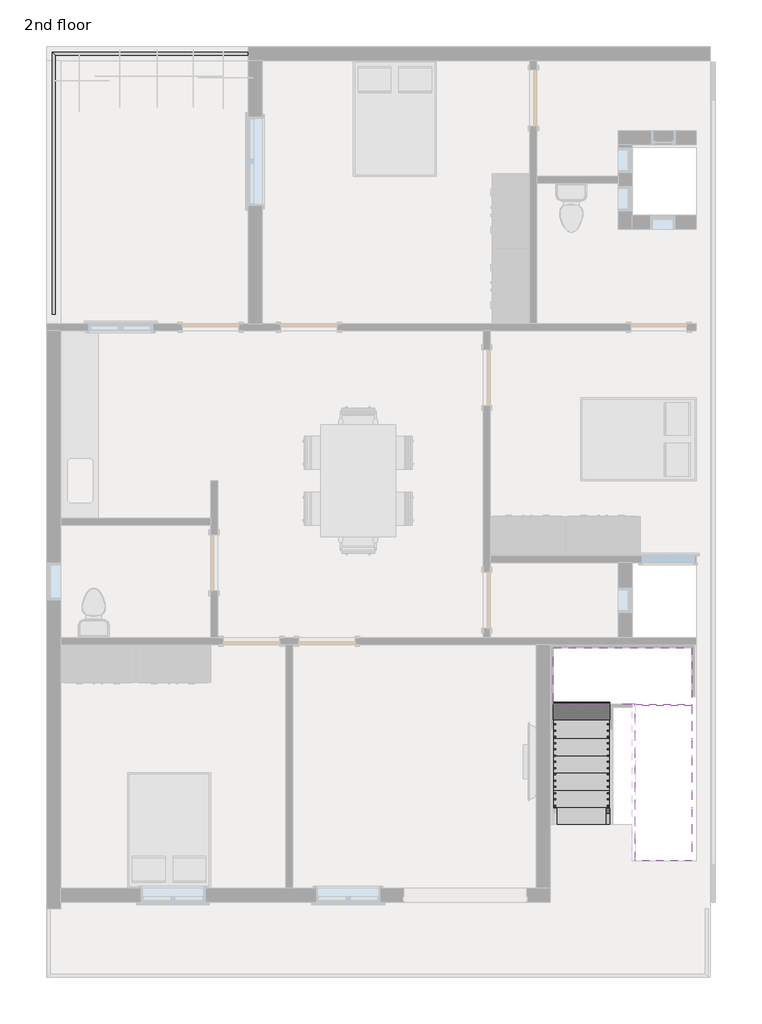
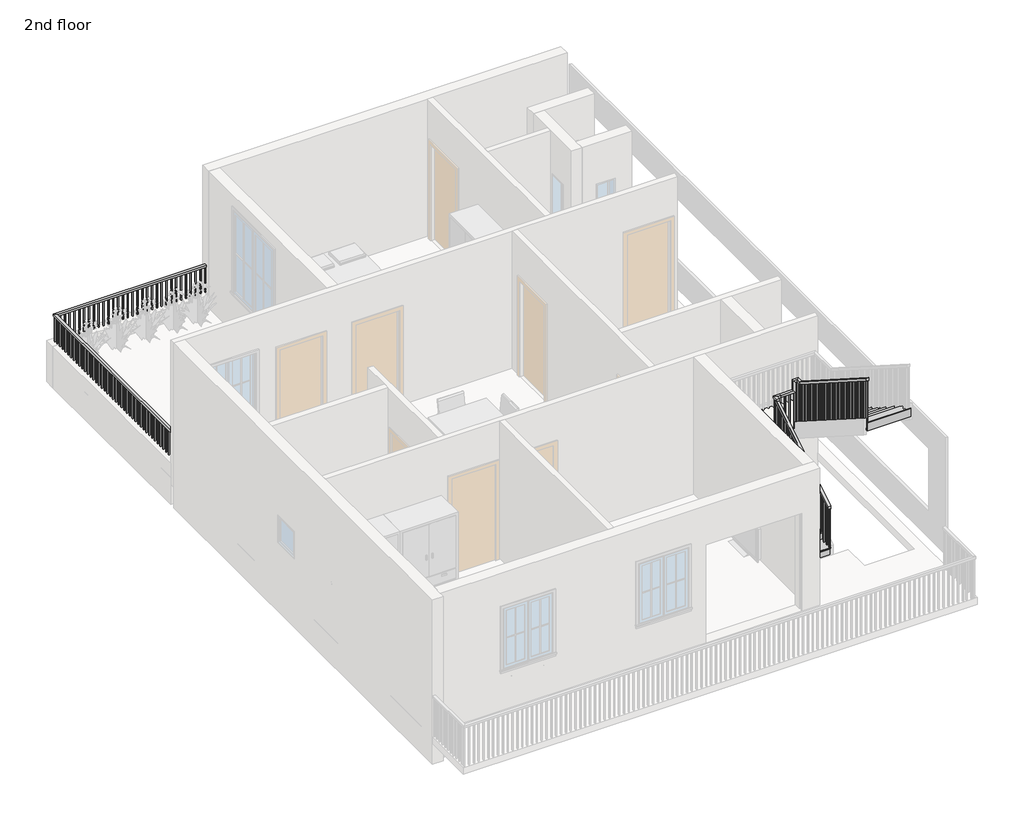
# One storey, part 3 of 5: 2 railings, 2 stair flights, 1 slab.
"""IFC4 building model written with IfcOpenShell, lengths in millimetres."""

from ifc_helpers import new_model, si_unit, frame, origin, place, context, project, spatial, polyline, outline, extrude, faceted_brep, transform, mapped, element, save
from components import non_monolithic_landing_99b9b51a, stair_flight_e21d000d, stair_flight_364c9dde

model = new_model("IFC4")

# Units and contexts
model_context = context("Model", 3, world=origin())
ifc_project = project(units=[si_unit("LENGTHUNIT", "METRE", prefix="MILLI")], contexts=[model_context])

# Site, building, storey
site = spatial("IfcSite", under=ifc_project)
building = spatial("IfcBuilding", under=site)
storey = spatial("IfcBuildingStorey", under=building, Name="2nd floor", Elevation=7010.4)

# Railings
placement = place(None, origin())
element("IfcRailing", 1, ObjectType="Handrail - Rectangular", at=placement, inside=storey, context=model_context, shape_type="SolidModel", body=[
    faceted_brep([(995.5501403, 157.6257925, 8102.6), (995.5501403, 157.6257925, 8042.386276), (1046.3501403, 157.6257925, 8042.386276), (1046.3501403, 157.6257925, 8102.6), (995.5501403, 2037.2257925, 9298.7090909), (995.5501403, 2088.0257925, 9270.8226396), (1046.3501403, 2088.0257925, 9270.8226396), (1046.3501403, 2037.2257925, 9298.7090909), (995.5501403, 2037.2257925, 9347.2), (995.5501403, 2088.0257925, 9296.4), (1046.3501403, 2088.0257925, 9296.4), (1046.3501403, 2037.2257925, 9347.2), (995.5501403, 2164.2257925, 9347.2), (995.5501403, 2164.2257925, 9296.4), (1046.3501403, 2113.4257925, 9296.4), (1046.3501403, 2113.4257925, 9347.2), (1122.5501403, 2164.2257925, 9347.2), (1122.5501403, 2164.2257925, 9296.4), (1122.5501403, 2113.4257925, 9296.4), (1122.5501403, 2113.4257925, 9347.2), (1389.2501403, 2164.2257925, 9347.2), (1440.0501403, 2164.2257925, 9296.4), (1440.0501403, 2113.4257925, 9296.4), (1389.2501403, 2113.4257925, 9347.2), (1389.2501403, 2164.2257925, 9573.4909091), (1440.0501403, 2164.2257925, 9522.6909091), (1440.0501403, 2113.4257925, 9522.6909091), (1389.2501403, 2113.4257925, 9573.4909091), (1516.2501403, 2164.2257925, 9573.4909091), (1516.2501403, 2164.2257925, 9522.6909091), (1465.4501403, 2113.4257925, 9522.6909091), (1465.4501403, 2113.4257925, 9573.4909091), (1516.2501403, 2037.2257925, 9573.4909091), (1516.2501403, 2022.4327976, 9522.6909091), (1465.4501403, 2022.4327976, 9522.6909091), (1465.4501403, 2037.2257925, 9573.4909091), (1516.2501403, -401.1742075, 11125.2), (1465.4501403, -401.1742075, 11125.2), (1465.4501403, -401.1742075, 11064.986276), (1516.2501403, -401.1742075, 11064.986276)], [[[0, 1, 2, 3]], [[1, 0, 4, 5]], [[2, 1, 5, 6]], [[3, 2, 6, 7]], [[0, 3, 7, 4]], [[5, 4, 8, 9]], [[6, 5, 9, 10]], [[7, 6, 10, 11]], [[4, 7, 11, 8]], [[9, 8, 12, 13]], [[10, 9, 13, 14]], [[11, 10, 14, 15]], [[8, 11, 15, 12]], [[13, 12, 16, 17]], [[14, 13, 17, 18]], [[15, 14, 18, 19]], [[12, 15, 19, 16]], [[17, 16, 20, 21]], [[18, 17, 21, 22]], [[19, 18, 22, 23]], [[16, 19, 23, 20]], [[21, 20, 24, 25]], [[22, 21, 25, 26]], [[23, 22, 26, 27]], [[20, 23, 27, 24]], [[25, 24, 28, 29]], [[26, 25, 29, 30]], [[27, 26, 30, 31]], [[24, 27, 31, 28]], [[29, 28, 32, 33]], [[30, 29, 33, 34]], [[31, 30, 34, 35]], [[28, 31, 35, 32]], [[36, 37, 38, 39]], [[33, 32, 36, 39]], [[34, 33, 39, 38]], [[35, 34, 38, 37]], [[32, 35, 37, 36]]]),
    extrude(outline(polyline([(-309.0992075, 11006.3930941), (-290.0492075, 10994.2703669), (-290.0492075, 10033.0), (-309.0992075, 10033.0), (-309.0992075, 11006.3930941)])), frame((1481.3251403, 0.0, 0.0), z_axis=(1.0, 0.0, 0.0), x_axis=(0.0, 1.0, 0.0)), (0.0, 0.0, 1.0), 19.05),
    extrude(outline(polyline([(-207.4992075, 10941.7385487), (-188.4492075, 10929.6158214), (-188.4492075, 10033.0), (-207.4992075, 10033.0), (-207.4992075, 10941.7385487)])), frame((1481.3251403, 0.0, 0.0), z_axis=(1.0, 0.0, 0.0), x_axis=(0.0, 1.0, 0.0)), (0.0, 0.0, 1.0), 19.05),
    extrude(outline(polyline([(-105.8992075, 10877.0840032), (-86.8492075, 10864.961276), (-86.8492075, 9855.2), (-105.8992075, 9855.2), (-105.8992075, 10877.0840032)])), frame((1481.3251403, 0.0, 0.0), z_axis=(1.0, 0.0, 0.0), x_axis=(0.0, 1.0, 0.0)), (0.0, 0.0, 1.0), 19.05),
    extrude(outline(polyline([(-4.2992075, 10812.4294578), (14.7507925, 10800.3067305), (14.7507925, 9855.2), (-4.2992075, 9855.2), (-4.2992075, 10812.4294578)])), frame((1481.3251403, 0.0, 0.0), z_axis=(1.0, 0.0, 0.0), x_axis=(0.0, 1.0, 0.0)), (0.0, 0.0, 1.0), 19.05),
    extrude(outline(polyline([(97.3007925, 10747.7749123), (116.3507925, 10735.6521851), (116.3507925, 9855.2), (97.3007925, 9855.2), (97.3007925, 10747.7749123)])), frame((1481.3251403, 0.0, 0.0), z_axis=(1.0, 0.0, 0.0), x_axis=(0.0, 1.0, 0.0)), (0.0, 0.0, 1.0), 19.05),
    extrude(outline(polyline([(198.9007925, 10683.1203669), (217.9507925, 10670.9976396), (217.9507925, 9677.4), (198.9007925, 9677.4), (198.9007925, 10683.1203669)])), frame((1481.3251403, 0.0, 0.0), z_axis=(1.0, 0.0, 0.0), x_axis=(0.0, 1.0, 0.0)), (0.0, 0.0, 1.0), 19.05),
    extrude(outline(polyline([(300.5007925, 10618.4658214), (319.5507925, 10606.3430941), (319.5507925, 9677.4), (300.5007925, 9677.4), (300.5007925, 10618.4658214)])), frame((1481.3251403, 0.0, 0.0), z_axis=(1.0, 0.0, 0.0), x_axis=(0.0, 1.0, 0.0)), (0.0, 0.0, 1.0), 19.05),
    extrude(outline(polyline([(402.1007925, 10553.811276), (421.1507925, 10541.6885487), (421.1507925, 9677.4), (402.1007925, 9677.4), (402.1007925, 10553.811276)])), frame((1481.3251403, 0.0, 0.0), z_axis=(1.0, 0.0, 0.0), x_axis=(0.0, 1.0, 0.0)), (0.0, 0.0, 1.0), 19.05),
    extrude(outline(polyline([(503.7007925, 10489.1567305), (522.7507925, 10477.0340032), (522.7507925, 9499.6), (503.7007925, 9499.6), (503.7007925, 10489.1567305)])), frame((1481.3251403, 0.0, 0.0), z_axis=(1.0, 0.0, 0.0), x_axis=(0.0, 1.0, 0.0)), (0.0, 0.0, 1.0), 19.05),
    extrude(outline(polyline([(605.3007925, 10424.5021851), (624.3507925, 10412.3794578), (624.3507925, 9499.6), (605.3007925, 9499.6), (605.3007925, 10424.5021851)])), frame((1481.3251403, 0.0, 0.0), z_axis=(1.0, 0.0, 0.0), x_axis=(0.0, 1.0, 0.0)), (0.0, 0.0, 1.0), 19.05),
    extrude(outline(polyline([(706.9007925, 10359.8476396), (725.9507925, 10347.7249123), (725.9507925, 9499.6), (706.9007925, 9499.6), (706.9007925, 10359.8476396)])), frame((1481.3251403, 0.0, 0.0), z_axis=(1.0, 0.0, 0.0), x_axis=(0.0, 1.0, 0.0)), (0.0, 0.0, 1.0), 19.05),
    extrude(outline(polyline([(808.5007925, 10295.1930941), (827.5507925, 10283.0703669), (827.5507925, 9321.8), (808.5007925, 9321.8), (808.5007925, 10295.1930941)])), frame((1481.3251403, 0.0, 0.0), z_axis=(1.0, 0.0, 0.0), x_axis=(0.0, 1.0, 0.0)), (0.0, 0.0, 1.0), 19.05),
    extrude(outline(polyline([(910.1007925, 10230.5385487), (929.1507925, 10218.4158214), (929.1507925, 9321.8), (910.1007925, 9321.8), (910.1007925, 10230.5385487)])), frame((1481.3251403, 0.0, 0.0), z_axis=(1.0, 0.0, 0.0), x_axis=(0.0, 1.0, 0.0)), (0.0, 0.0, 1.0), 19.05),
    extrude(outline(polyline([(1011.7007925, 10165.8840032), (1030.7507925, 10153.761276), (1030.7507925, 9144.0), (1011.7007925, 9144.0), (1011.7007925, 10165.8840032)])), frame((1481.3251403, 0.0, 0.0), z_axis=(1.0, 0.0, 0.0), x_axis=(0.0, 1.0, 0.0)), (0.0, 0.0, 1.0), 19.05),
    extrude(outline(polyline([(1113.3007925, 10101.2294578), (1132.3507925, 10089.1067305), (1132.3507925, 9144.0), (1113.3007925, 9144.0), (1113.3007925, 10101.2294578)])), frame((1481.3251403, 0.0, 0.0), z_axis=(1.0, 0.0, 0.0), x_axis=(0.0, 1.0, 0.0)), (0.0, 0.0, 1.0), 19.05),
    extrude(outline(polyline([(1214.9007925, 10036.5749123), (1233.9507925, 10024.4521851), (1233.9507925, 9144.0), (1214.9007925, 9144.0), (1214.9007925, 10036.5749123)])), frame((1481.3251403, 0.0, 0.0), z_axis=(1.0, 0.0, 0.0), x_axis=(0.0, 1.0, 0.0)), (0.0, 0.0, 1.0), 19.05),
    extrude(outline(polyline([(1316.5007925, 9971.9203669), (1335.5507925, 9959.7976396), (1335.5507925, 8966.2), (1316.5007925, 8966.2), (1316.5007925, 9971.9203669)])), frame((1481.3251403, 0.0, 0.0), z_axis=(1.0, 0.0, 0.0), x_axis=(0.0, 1.0, 0.0)), (0.0, 0.0, 1.0), 19.05),
    extrude(outline(polyline([(1418.1007925, 9907.2658214), (1437.1507925, 9895.1430941), (1437.1507925, 8966.2), (1418.1007925, 8966.2), (1418.1007925, 9907.2658214)])), frame((1481.3251403, 0.0, 0.0), z_axis=(1.0, 0.0, 0.0), x_axis=(0.0, 1.0, 0.0)), (0.0, 0.0, 1.0), 19.05),
    extrude(outline(polyline([(1519.7007925, 9842.611276), (1538.7507925, 9830.4885487), (1538.7507925, 8966.2), (1519.7007925, 8966.2), (1519.7007925, 9842.611276)])), frame((1481.3251403, 0.0, 0.0), z_axis=(1.0, 0.0, 0.0), x_axis=(0.0, 1.0, 0.0)), (0.0, 0.0, 1.0), 19.05),
    extrude(outline(polyline([(1621.3007925, 9777.9567305), (1640.3507925, 9765.8340032), (1640.3507925, 8788.4), (1621.3007925, 8788.4), (1621.3007925, 9777.9567305)])), frame((1481.3251403, 0.0, 0.0), z_axis=(1.0, 0.0, 0.0), x_axis=(0.0, 1.0, 0.0)), (0.0, 0.0, 1.0), 19.05),
    extrude(outline(polyline([(1722.9007925, 9713.3021851), (1741.9507925, 9701.1794578), (1741.9507925, 8788.4), (1722.9007925, 8788.4), (1722.9007925, 9713.3021851)])), frame((1481.3251403, 0.0, 0.0), z_axis=(1.0, 0.0, 0.0), x_axis=(0.0, 1.0, 0.0)), (0.0, 0.0, 1.0), 19.05),
    extrude(outline(polyline([(1824.5007925, 9648.6476396), (1843.5507925, 9636.5249123), (1843.5507925, 8788.4), (1824.5007925, 8788.4), (1824.5007925, 9648.6476396)])), frame((1481.3251403, 0.0, 0.0), z_axis=(1.0, 0.0, 0.0), x_axis=(0.0, 1.0, 0.0)), (0.0, 0.0, 1.0), 19.05),
    extrude(outline(polyline([(1926.1007925, 9583.9930941), (1945.1507925, 9571.8703669), (1945.1507925, 8610.6), (1926.1007925, 8610.6), (1926.1007925, 9583.9930941)])), frame((1481.3251403, 0.0, 0.0), z_axis=(1.0, 0.0, 0.0), x_axis=(0.0, 1.0, 0.0)), (0.0, 0.0, 1.0), 19.05),
    extrude(outline(polyline([(2027.7007925, 9519.3385487), (2046.7507925, 9507.2158214), (2046.7507925, 8610.6), (2027.7007925, 8610.6), (2027.7007925, 9519.3385487)])), frame((1481.3251403, 0.0, 0.0), z_axis=(1.0, 0.0, 0.0), x_axis=(0.0, 1.0, 0.0)), (0.0, 0.0, 1.0), 19.05),
    extrude(outline(polyline([(1417.8251403, 2129.3007925), (1417.8251403, 2148.3507925), (1436.8751403, 2148.3507925), (1436.8751403, 2129.3007925), (1417.8251403, 2129.3007925)])), frame((0.0, 0.0, 8432.8), z_axis=(0.0, 0.0, 1.0), x_axis=(1.0, 0.0, 0.0)), (0.0, 0.0, 1.0), 1089.8909091),
    extrude(outline(polyline([(1316.2251403, 2129.3007925), (1316.2251403, 2148.3507925), (1335.2751403, 2148.3507925), (1335.2751403, 2129.3007925), (1316.2251403, 2129.3007925)])), frame((0.0, 0.0, 8432.8), z_axis=(0.0, 0.0, 1.0), x_axis=(1.0, 0.0, 0.0)), (0.0, 0.0, 1.0), 863.6),
    extrude(outline(polyline([(1214.6251403, 2129.3007925), (1214.6251403, 2148.3507925), (1233.6751403, 2148.3507925), (1233.6751403, 2129.3007925), (1214.6251403, 2129.3007925)])), frame((0.0, 0.0, 8432.8), z_axis=(0.0, 0.0, 1.0), x_axis=(1.0, 0.0, 0.0)), (0.0, 0.0, 1.0), 863.6),
    extrude(outline(polyline([(1113.0251403, 2129.3007925), (1113.0251403, 2148.3507925), (1132.0751403, 2148.3507925), (1132.0751403, 2129.3007925), (1113.0251403, 2129.3007925)])), frame((0.0, 0.0, 8432.8), z_axis=(0.0, 0.0, 1.0), x_axis=(1.0, 0.0, 0.0)), (0.0, 0.0, 1.0), 863.6),
    extrude(outline(polyline([(1030.4751403, 2078.5007925), (1011.4251403, 2078.5007925), (1011.4251403, 2097.5507925), (1030.4751403, 2097.5507925), (1030.4751403, 2078.5007925)])), frame((0.0, 0.0, 8255.0), z_axis=(0.0, 0.0, 1.0), x_axis=(1.0, 0.0, 0.0)), (0.0, 0.0, 1.0), 1041.4),
    extrude(outline(polyline([(1976.9007925, 9200.1067305), (1995.9507925, 9212.2294578), (1995.9507925, 8255.0), (1976.9007925, 8255.0), (1976.9007925, 9200.1067305)])), frame((1011.4251403, 0.0, 0.0), z_axis=(1.0, 0.0, 0.0), x_axis=(0.0, 1.0, 0.0)), (0.0, 0.0, 1.0), 19.05),
    extrude(outline(polyline([(1875.3007925, 9135.4521851), (1894.3507925, 9147.5749123), (1894.3507925, 8255.0), (1875.3007925, 8255.0), (1875.3007925, 9135.4521851)])), frame((1011.4251403, 0.0, 0.0), z_axis=(1.0, 0.0, 0.0), x_axis=(0.0, 1.0, 0.0)), (0.0, 0.0, 1.0), 19.05),
    extrude(outline(polyline([(1773.7007925, 9070.7976396), (1792.7507925, 9082.9203669), (1792.7507925, 8077.2), (1773.7007925, 8077.2), (1773.7007925, 9070.7976396)])), frame((1011.4251403, 0.0, 0.0), z_axis=(1.0, 0.0, 0.0), x_axis=(0.0, 1.0, 0.0)), (0.0, 0.0, 1.0), 19.05),
    extrude(outline(polyline([(1672.1007925, 9006.1430941), (1691.1507925, 9018.2658214), (1691.1507925, 8077.2), (1672.1007925, 8077.2), (1672.1007925, 9006.1430941)])), frame((1011.4251403, 0.0, 0.0), z_axis=(1.0, 0.0, 0.0), x_axis=(0.0, 1.0, 0.0)), (0.0, 0.0, 1.0), 19.05),
    extrude(outline(polyline([(1570.5007925, 8941.4885487), (1589.5507925, 8953.611276), (1589.5507925, 8077.2), (1570.5007925, 8077.2), (1570.5007925, 8941.4885487)])), frame((1011.4251403, 0.0, 0.0), z_axis=(1.0, 0.0, 0.0), x_axis=(0.0, 1.0, 0.0)), (0.0, 0.0, 1.0), 19.05),
    extrude(outline(polyline([(1468.9007925, 8876.8340032), (1487.9507925, 8888.9567305), (1487.9507925, 7899.4), (1468.9007925, 7899.4), (1468.9007925, 8876.8340032)])), frame((1011.4251403, 0.0, 0.0), z_axis=(1.0, 0.0, 0.0), x_axis=(0.0, 1.0, 0.0)), (0.0, 0.0, 1.0), 19.05),
    extrude(outline(polyline([(1367.3007925, 8812.1794578), (1386.3507925, 8824.3021851), (1386.3507925, 7899.4), (1367.3007925, 7899.4), (1367.3007925, 8812.1794578)])), frame((1011.4251403, 0.0, 0.0), z_axis=(1.0, 0.0, 0.0), x_axis=(0.0, 1.0, 0.0)), (0.0, 0.0, 1.0), 19.05),
    extrude(outline(polyline([(1265.7007925, 8747.5249123), (1284.7507925, 8759.6476396), (1284.7507925, 7899.4), (1265.7007925, 7899.4), (1265.7007925, 8747.5249123)])), frame((1011.4251403, 0.0, 0.0), z_axis=(1.0, 0.0, 0.0), x_axis=(0.0, 1.0, 0.0)), (0.0, 0.0, 1.0), 19.05),
    extrude(outline(polyline([(1164.1007925, 8682.8703669), (1183.1507925, 8694.9930941), (1183.1507925, 7721.6), (1164.1007925, 7721.6), (1164.1007925, 8682.8703669)])), frame((1011.4251403, 0.0, 0.0), z_axis=(1.0, 0.0, 0.0), x_axis=(0.0, 1.0, 0.0)), (0.0, 0.0, 1.0), 19.05),
    extrude(outline(polyline([(1062.5007925, 8618.2158214), (1081.5507925, 8630.3385487), (1081.5507925, 7721.6), (1062.5007925, 7721.6), (1062.5007925, 8618.2158214)])), frame((1011.4251403, 0.0, 0.0), z_axis=(1.0, 0.0, 0.0), x_axis=(0.0, 1.0, 0.0)), (0.0, 0.0, 1.0), 19.05),
    extrude(outline(polyline([(960.9007925, 8553.561276), (979.9507925, 8565.6840032), (979.9507925, 7543.8), (960.9007925, 7543.8), (960.9007925, 8553.561276)])), frame((1011.4251403, 0.0, 0.0), z_axis=(1.0, 0.0, 0.0), x_axis=(0.0, 1.0, 0.0)), (0.0, 0.0, 1.0), 19.05),
    extrude(outline(polyline([(859.3007925, 8488.9067305), (878.3507925, 8501.0294578), (878.3507925, 7543.8), (859.3007925, 7543.8), (859.3007925, 8488.9067305)])), frame((1011.4251403, 0.0, 0.0), z_axis=(1.0, 0.0, 0.0), x_axis=(0.0, 1.0, 0.0)), (0.0, 0.0, 1.0), 19.05),
    extrude(outline(polyline([(757.7007925, 8424.2521851), (776.7507925, 8436.3749123), (776.7507925, 7543.8), (757.7007925, 7543.8), (757.7007925, 8424.2521851)])), frame((1011.4251403, 0.0, 0.0), z_axis=(1.0, 0.0, 0.0), x_axis=(0.0, 1.0, 0.0)), (0.0, 0.0, 1.0), 19.05),
    extrude(outline(polyline([(656.1007925, 8359.5976396), (675.1507925, 8371.7203669), (675.1507925, 7366.0), (656.1007925, 7366.0), (656.1007925, 8359.5976396)])), frame((1011.4251403, 0.0, 0.0), z_axis=(1.0, 0.0, 0.0), x_axis=(0.0, 1.0, 0.0)), (0.0, 0.0, 1.0), 19.05),
    extrude(outline(polyline([(554.5007925, 8294.9430941), (573.5507925, 8307.0658214), (573.5507925, 7366.0), (554.5007925, 7366.0), (554.5007925, 8294.9430941)])), frame((1011.4251403, 0.0, 0.0), z_axis=(1.0, 0.0, 0.0), x_axis=(0.0, 1.0, 0.0)), (0.0, 0.0, 1.0), 19.05),
    extrude(outline(polyline([(452.9007925, 8230.2885487), (471.9507925, 8242.411276), (471.9507925, 7366.0), (452.9007925, 7366.0), (452.9007925, 8230.2885487)])), frame((1011.4251403, 0.0, 0.0), z_axis=(1.0, 0.0, 0.0), x_axis=(0.0, 1.0, 0.0)), (0.0, 0.0, 1.0), 19.05),
    extrude(outline(polyline([(351.3007925, 8165.6340032), (370.3507925, 8177.7567305), (370.3507925, 7188.2), (351.3007925, 7188.2), (351.3007925, 8165.6340032)])), frame((1011.4251403, 0.0, 0.0), z_axis=(1.0, 0.0, 0.0), x_axis=(0.0, 1.0, 0.0)), (0.0, 0.0, 1.0), 19.05),
    extrude(outline(polyline([(249.7007925, 8100.9794578), (268.7507925, 8113.1021851), (268.7507925, 7188.2), (249.7007925, 7188.2), (249.7007925, 8100.9794578)])), frame((1011.4251403, 0.0, 0.0), z_axis=(1.0, 0.0, 0.0), x_axis=(0.0, 1.0, 0.0)), (0.0, 0.0, 1.0), 19.05),
    extrude(outline(polyline([(1481.3251403, 2129.3007925), (1481.3251403, 2148.3507925), (1500.3751403, 2148.3507925), (1500.3751403, 2129.3007925), (1481.3251403, 2129.3007925)])), frame((0.0, 0.0, 8432.8), z_axis=(0.0, 0.0, 1.0), x_axis=(1.0, 0.0, 0.0)), (0.0, 0.0, 1.0), 1089.8909091),
    extrude(outline(polyline([(1030.4751403, 2129.3007925), (1011.4251403, 2129.3007925), (1011.4251403, 2148.3507925), (1030.4751403, 2148.3507925), (1030.4751403, 2129.3007925)])), frame((0.0, 0.0, 8432.8), z_axis=(0.0, 0.0, 1.0), x_axis=(1.0, 0.0, 0.0)), (0.0, 0.0, 1.0), 863.6),
    extrude(outline(polyline([(-401.1742075, 11064.986276), (-382.1242075, 11052.8635487), (-382.1242075, 10033.0), (-401.1742075, 10033.0), (-401.1742075, 11064.986276)])), frame((1481.3251403, 0.0, 0.0), z_axis=(1.0, 0.0, 0.0), x_axis=(0.0, 1.0, 0.0)), (0.0, 0.0, 1.0), 19.05),
    extrude(outline(polyline([(157.6257925, 8042.386276), (176.6757925, 8054.5090032), (176.6757925, 7188.2), (157.6257925, 7188.2), (157.6257925, 8042.386276)])), frame((1011.4251403, 0.0, 0.0), z_axis=(1.0, 0.0, 0.0), x_axis=(0.0, 1.0, 0.0)), (0.0, 0.0, 1.0), 19.05),
])
element("IfcRailing", 2, ObjectType="Handrail - Rectangular", at=placement, inside=storey, context=model_context, shape_type="SolidModel", body=[
    faceted_brep([(-8021.4498597, 8450.7257925, 7924.8), (-8021.4498597, 8450.7257925, 7874.0), (-7970.6498597, 8450.7257925, 7874.0), (-7970.6498597, 8450.7257925, 7924.8), (-8021.4498597, 12717.9257925, 7924.8), (-8021.4498597, 12717.9257925, 7874.0), (-7970.6498597, 12667.1257925, 7874.0), (-7970.6498597, 12667.1257925, 7924.8), (-4795.6498597, 12717.9257925, 7924.8), (-4795.6498597, 12667.1257925, 7924.8), (-4795.6498597, 12667.1257925, 7874.0), (-4795.6498597, 12717.9257925, 7874.0)], [[[0, 1, 2, 3]], [[1, 0, 4, 5]], [[2, 1, 5, 6]], [[3, 2, 6, 7]], [[0, 3, 7, 4]], [[8, 9, 10, 11]], [[5, 4, 8, 11]], [[6, 5, 11, 10]], [[7, 6, 10, 9]], [[4, 7, 9, 8]]]),
    extrude(outline(polyline([(-4855.9748597, 12683.0007925), (-4855.9748597, 12702.0507925), (-4836.9248597, 12702.0507925), (-4836.9248597, 12683.0007925), (-4855.9748597, 12683.0007925)])), frame((0.0, 0.0, 7010.4), z_axis=(0.0, 0.0, 1.0), x_axis=(1.0, 0.0, 0.0)), (0.0, 0.0, 1.0), 863.6),
    extrude(outline(polyline([(-4957.5748597, 12683.0007925), (-4957.5748597, 12702.0507925), (-4938.5248597, 12702.0507925), (-4938.5248597, 12683.0007925), (-4957.5748597, 12683.0007925)])), frame((0.0, 0.0, 7010.4), z_axis=(0.0, 0.0, 1.0), x_axis=(1.0, 0.0, 0.0)), (0.0, 0.0, 1.0), 863.6),
    extrude(outline(polyline([(-5059.1748597, 12683.0007925), (-5059.1748597, 12702.0507925), (-5040.1248597, 12702.0507925), (-5040.1248597, 12683.0007925), (-5059.1748597, 12683.0007925)])), frame((0.0, 0.0, 7010.4), z_axis=(0.0, 0.0, 1.0), x_axis=(1.0, 0.0, 0.0)), (0.0, 0.0, 1.0), 863.6),
    extrude(outline(polyline([(-5160.7748597, 12683.0007925), (-5160.7748597, 12702.0507925), (-5141.7248597, 12702.0507925), (-5141.7248597, 12683.0007925), (-5160.7748597, 12683.0007925)])), frame((0.0, 0.0, 7010.4), z_axis=(0.0, 0.0, 1.0), x_axis=(1.0, 0.0, 0.0)), (0.0, 0.0, 1.0), 863.6),
    extrude(outline(polyline([(-5262.3748597, 12683.0007925), (-5262.3748597, 12702.0507925), (-5243.3248597, 12702.0507925), (-5243.3248597, 12683.0007925), (-5262.3748597, 12683.0007925)])), frame((0.0, 0.0, 7010.4), z_axis=(0.0, 0.0, 1.0), x_axis=(1.0, 0.0, 0.0)), (0.0, 0.0, 1.0), 863.6),
    extrude(outline(polyline([(-5363.9748597, 12683.0007925), (-5363.9748597, 12702.0507925), (-5344.9248597, 12702.0507925), (-5344.9248597, 12683.0007925), (-5363.9748597, 12683.0007925)])), frame((0.0, 0.0, 7010.4), z_axis=(0.0, 0.0, 1.0), x_axis=(1.0, 0.0, 0.0)), (0.0, 0.0, 1.0), 863.6),
    extrude(outline(polyline([(-5465.5748597, 12683.0007925), (-5465.5748597, 12702.0507925), (-5446.5248597, 12702.0507925), (-5446.5248597, 12683.0007925), (-5465.5748597, 12683.0007925)])), frame((0.0, 0.0, 7010.4), z_axis=(0.0, 0.0, 1.0), x_axis=(1.0, 0.0, 0.0)), (0.0, 0.0, 1.0), 863.6),
    extrude(outline(polyline([(-5567.1748597, 12683.0007925), (-5567.1748597, 12702.0507925), (-5548.1248597, 12702.0507925), (-5548.1248597, 12683.0007925), (-5567.1748597, 12683.0007925)])), frame((0.0, 0.0, 7010.4), z_axis=(0.0, 0.0, 1.0), x_axis=(1.0, 0.0, 0.0)), (0.0, 0.0, 1.0), 863.6),
    extrude(outline(polyline([(-5668.7748597, 12683.0007925), (-5668.7748597, 12702.0507925), (-5649.7248597, 12702.0507925), (-5649.7248597, 12683.0007925), (-5668.7748597, 12683.0007925)])), frame((0.0, 0.0, 7010.4), z_axis=(0.0, 0.0, 1.0), x_axis=(1.0, 0.0, 0.0)), (0.0, 0.0, 1.0), 863.6),
    extrude(outline(polyline([(-5770.3748597, 12683.0007925), (-5770.3748597, 12702.0507925), (-5751.3248597, 12702.0507925), (-5751.3248597, 12683.0007925), (-5770.3748597, 12683.0007925)])), frame((0.0, 0.0, 7010.4), z_axis=(0.0, 0.0, 1.0), x_axis=(1.0, 0.0, 0.0)), (0.0, 0.0, 1.0), 863.6),
    extrude(outline(polyline([(-5871.9748597, 12683.0007925), (-5871.9748597, 12702.0507925), (-5852.9248597, 12702.0507925), (-5852.9248597, 12683.0007925), (-5871.9748597, 12683.0007925)])), frame((0.0, 0.0, 7010.4), z_axis=(0.0, 0.0, 1.0), x_axis=(1.0, 0.0, 0.0)), (0.0, 0.0, 1.0), 863.6),
    extrude(outline(polyline([(-5973.5748597, 12683.0007925), (-5973.5748597, 12702.0507925), (-5954.5248597, 12702.0507925), (-5954.5248597, 12683.0007925), (-5973.5748597, 12683.0007925)])), frame((0.0, 0.0, 7010.4), z_axis=(0.0, 0.0, 1.0), x_axis=(1.0, 0.0, 0.0)), (0.0, 0.0, 1.0), 863.6),
    extrude(outline(polyline([(-6075.1748597, 12683.0007925), (-6075.1748597, 12702.0507925), (-6056.1248597, 12702.0507925), (-6056.1248597, 12683.0007925), (-6075.1748597, 12683.0007925)])), frame((0.0, 0.0, 7010.4), z_axis=(0.0, 0.0, 1.0), x_axis=(1.0, 0.0, 0.0)), (0.0, 0.0, 1.0), 863.6),
    extrude(outline(polyline([(-6176.7748597, 12683.0007925), (-6176.7748597, 12702.0507925), (-6157.7248597, 12702.0507925), (-6157.7248597, 12683.0007925), (-6176.7748597, 12683.0007925)])), frame((0.0, 0.0, 7010.4), z_axis=(0.0, 0.0, 1.0), x_axis=(1.0, 0.0, 0.0)), (0.0, 0.0, 1.0), 863.6),
    extrude(outline(polyline([(-6278.3748597, 12683.0007925), (-6278.3748597, 12702.0507925), (-6259.3248597, 12702.0507925), (-6259.3248597, 12683.0007925), (-6278.3748597, 12683.0007925)])), frame((0.0, 0.0, 7010.4), z_axis=(0.0, 0.0, 1.0), x_axis=(1.0, 0.0, 0.0)), (0.0, 0.0, 1.0), 863.6),
    extrude(outline(polyline([(-6379.9748597, 12683.0007925), (-6379.9748597, 12702.0507925), (-6360.9248597, 12702.0507925), (-6360.9248597, 12683.0007925), (-6379.9748597, 12683.0007925)])), frame((0.0, 0.0, 7010.4), z_axis=(0.0, 0.0, 1.0), x_axis=(1.0, 0.0, 0.0)), (0.0, 0.0, 1.0), 863.6),
    extrude(outline(polyline([(-6481.5748597, 12683.0007925), (-6481.5748597, 12702.0507925), (-6462.5248597, 12702.0507925), (-6462.5248597, 12683.0007925), (-6481.5748597, 12683.0007925)])), frame((0.0, 0.0, 7010.4), z_axis=(0.0, 0.0, 1.0), x_axis=(1.0, 0.0, 0.0)), (0.0, 0.0, 1.0), 863.6),
    extrude(outline(polyline([(-6583.1748597, 12683.0007925), (-6583.1748597, 12702.0507925), (-6564.1248597, 12702.0507925), (-6564.1248597, 12683.0007925), (-6583.1748597, 12683.0007925)])), frame((0.0, 0.0, 7010.4), z_axis=(0.0, 0.0, 1.0), x_axis=(1.0, 0.0, 0.0)), (0.0, 0.0, 1.0), 863.6),
    extrude(outline(polyline([(-6684.7748597, 12683.0007925), (-6684.7748597, 12702.0507925), (-6665.7248597, 12702.0507925), (-6665.7248597, 12683.0007925), (-6684.7748597, 12683.0007925)])), frame((0.0, 0.0, 7010.4), z_axis=(0.0, 0.0, 1.0), x_axis=(1.0, 0.0, 0.0)), (0.0, 0.0, 1.0), 863.6),
    extrude(outline(polyline([(-6786.3748597, 12683.0007925), (-6786.3748597, 12702.0507925), (-6767.3248597, 12702.0507925), (-6767.3248597, 12683.0007925), (-6786.3748597, 12683.0007925)])), frame((0.0, 0.0, 7010.4), z_axis=(0.0, 0.0, 1.0), x_axis=(1.0, 0.0, 0.0)), (0.0, 0.0, 1.0), 863.6),
    extrude(outline(polyline([(-6887.9748597, 12683.0007925), (-6887.9748597, 12702.0507925), (-6868.9248597, 12702.0507925), (-6868.9248597, 12683.0007925), (-6887.9748597, 12683.0007925)])), frame((0.0, 0.0, 7010.4), z_axis=(0.0, 0.0, 1.0), x_axis=(1.0, 0.0, 0.0)), (0.0, 0.0, 1.0), 863.6),
    extrude(outline(polyline([(-6989.5748597, 12683.0007925), (-6989.5748597, 12702.0507925), (-6970.5248597, 12702.0507925), (-6970.5248597, 12683.0007925), (-6989.5748597, 12683.0007925)])), frame((0.0, 0.0, 7010.4), z_axis=(0.0, 0.0, 1.0), x_axis=(1.0, 0.0, 0.0)), (0.0, 0.0, 1.0), 863.6),
    extrude(outline(polyline([(-7091.1748597, 12683.0007925), (-7091.1748597, 12702.0507925), (-7072.1248597, 12702.0507925), (-7072.1248597, 12683.0007925), (-7091.1748597, 12683.0007925)])), frame((0.0, 0.0, 7010.4), z_axis=(0.0, 0.0, 1.0), x_axis=(1.0, 0.0, 0.0)), (0.0, 0.0, 1.0), 863.6),
    extrude(outline(polyline([(-7192.7748597, 12683.0007925), (-7192.7748597, 12702.0507925), (-7173.7248597, 12702.0507925), (-7173.7248597, 12683.0007925), (-7192.7748597, 12683.0007925)])), frame((0.0, 0.0, 7010.4), z_axis=(0.0, 0.0, 1.0), x_axis=(1.0, 0.0, 0.0)), (0.0, 0.0, 1.0), 863.6),
    extrude(outline(polyline([(-7294.3748597, 12683.0007925), (-7294.3748597, 12702.0507925), (-7275.3248597, 12702.0507925), (-7275.3248597, 12683.0007925), (-7294.3748597, 12683.0007925)])), frame((0.0, 0.0, 7010.4), z_axis=(0.0, 0.0, 1.0), x_axis=(1.0, 0.0, 0.0)), (0.0, 0.0, 1.0), 863.6),
    extrude(outline(polyline([(-7395.9748597, 12683.0007925), (-7395.9748597, 12702.0507925), (-7376.9248597, 12702.0507925), (-7376.9248597, 12683.0007925), (-7395.9748597, 12683.0007925)])), frame((0.0, 0.0, 7010.4), z_axis=(0.0, 0.0, 1.0), x_axis=(1.0, 0.0, 0.0)), (0.0, 0.0, 1.0), 863.6),
    extrude(outline(polyline([(-7497.5748597, 12683.0007925), (-7497.5748597, 12702.0507925), (-7478.5248597, 12702.0507925), (-7478.5248597, 12683.0007925), (-7497.5748597, 12683.0007925)])), frame((0.0, 0.0, 7010.4), z_axis=(0.0, 0.0, 1.0), x_axis=(1.0, 0.0, 0.0)), (0.0, 0.0, 1.0), 863.6),
    extrude(outline(polyline([(-7599.1748597, 12683.0007925), (-7599.1748597, 12702.0507925), (-7580.1248597, 12702.0507925), (-7580.1248597, 12683.0007925), (-7599.1748597, 12683.0007925)])), frame((0.0, 0.0, 7010.4), z_axis=(0.0, 0.0, 1.0), x_axis=(1.0, 0.0, 0.0)), (0.0, 0.0, 1.0), 863.6),
    extrude(outline(polyline([(-7700.7748597, 12683.0007925), (-7700.7748597, 12702.0507925), (-7681.7248597, 12702.0507925), (-7681.7248597, 12683.0007925), (-7700.7748597, 12683.0007925)])), frame((0.0, 0.0, 7010.4), z_axis=(0.0, 0.0, 1.0), x_axis=(1.0, 0.0, 0.0)), (0.0, 0.0, 1.0), 863.6),
    extrude(outline(polyline([(-7802.3748597, 12683.0007925), (-7802.3748597, 12702.0507925), (-7783.3248597, 12702.0507925), (-7783.3248597, 12683.0007925), (-7802.3748597, 12683.0007925)])), frame((0.0, 0.0, 7010.4), z_axis=(0.0, 0.0, 1.0), x_axis=(1.0, 0.0, 0.0)), (0.0, 0.0, 1.0), 863.6),
    extrude(outline(polyline([(-7903.9748597, 12683.0007925), (-7903.9748597, 12702.0507925), (-7884.9248597, 12702.0507925), (-7884.9248597, 12683.0007925), (-7903.9748597, 12683.0007925)])), frame((0.0, 0.0, 7010.4), z_axis=(0.0, 0.0, 1.0), x_axis=(1.0, 0.0, 0.0)), (0.0, 0.0, 1.0), 863.6),
    extrude(outline(polyline([(-7986.5248597, 12606.8007925), (-8005.5748597, 12606.8007925), (-8005.5748597, 12625.8507925), (-7986.5248597, 12625.8507925), (-7986.5248597, 12606.8007925)])), frame((0.0, 0.0, 7010.4), z_axis=(0.0, 0.0, 1.0), x_axis=(1.0, 0.0, 0.0)), (0.0, 0.0, 1.0), 863.6),
    extrude(outline(polyline([(-7986.5248597, 12505.2007925), (-8005.5748597, 12505.2007925), (-8005.5748597, 12524.2507925), (-7986.5248597, 12524.2507925), (-7986.5248597, 12505.2007925)])), frame((0.0, 0.0, 7010.4), z_axis=(0.0, 0.0, 1.0), x_axis=(1.0, 0.0, 0.0)), (0.0, 0.0, 1.0), 863.6),
    extrude(outline(polyline([(-7986.5248597, 12403.6007925), (-8005.5748597, 12403.6007925), (-8005.5748597, 12422.6507925), (-7986.5248597, 12422.6507925), (-7986.5248597, 12403.6007925)])), frame((0.0, 0.0, 7010.4), z_axis=(0.0, 0.0, 1.0), x_axis=(1.0, 0.0, 0.0)), (0.0, 0.0, 1.0), 863.6),
    extrude(outline(polyline([(-7986.5248597, 12302.0007925), (-8005.5748597, 12302.0007925), (-8005.5748597, 12321.0507925), (-7986.5248597, 12321.0507925), (-7986.5248597, 12302.0007925)])), frame((0.0, 0.0, 7010.4), z_axis=(0.0, 0.0, 1.0), x_axis=(1.0, 0.0, 0.0)), (0.0, 0.0, 1.0), 863.6),
    extrude(outline(polyline([(-7986.5248597, 12200.4007925), (-8005.5748597, 12200.4007925), (-8005.5748597, 12219.4507925), (-7986.5248597, 12219.4507925), (-7986.5248597, 12200.4007925)])), frame((0.0, 0.0, 7010.4), z_axis=(0.0, 0.0, 1.0), x_axis=(1.0, 0.0, 0.0)), (0.0, 0.0, 1.0), 863.6),
    extrude(outline(polyline([(-7986.5248597, 12098.8007925), (-8005.5748597, 12098.8007925), (-8005.5748597, 12117.8507925), (-7986.5248597, 12117.8507925), (-7986.5248597, 12098.8007925)])), frame((0.0, 0.0, 7010.4), z_axis=(0.0, 0.0, 1.0), x_axis=(1.0, 0.0, 0.0)), (0.0, 0.0, 1.0), 863.6),
    extrude(outline(polyline([(-7986.5248597, 11997.2007925), (-8005.5748597, 11997.2007925), (-8005.5748597, 12016.2507925), (-7986.5248597, 12016.2507925), (-7986.5248597, 11997.2007925)])), frame((0.0, 0.0, 7010.4), z_axis=(0.0, 0.0, 1.0), x_axis=(1.0, 0.0, 0.0)), (0.0, 0.0, 1.0), 863.6),
    extrude(outline(polyline([(-7986.5248597, 11895.6007925), (-8005.5748597, 11895.6007925), (-8005.5748597, 11914.6507925), (-7986.5248597, 11914.6507925), (-7986.5248597, 11895.6007925)])), frame((0.0, 0.0, 7010.4), z_axis=(0.0, 0.0, 1.0), x_axis=(1.0, 0.0, 0.0)), (0.0, 0.0, 1.0), 863.6),
    extrude(outline(polyline([(-7986.5248597, 11794.0007925), (-8005.5748597, 11794.0007925), (-8005.5748597, 11813.0507925), (-7986.5248597, 11813.0507925), (-7986.5248597, 11794.0007925)])), frame((0.0, 0.0, 7010.4), z_axis=(0.0, 0.0, 1.0), x_axis=(1.0, 0.0, 0.0)), (0.0, 0.0, 1.0), 863.6),
    extrude(outline(polyline([(-7986.5248597, 11692.4007925), (-8005.5748597, 11692.4007925), (-8005.5748597, 11711.4507925), (-7986.5248597, 11711.4507925), (-7986.5248597, 11692.4007925)])), frame((0.0, 0.0, 7010.4), z_axis=(0.0, 0.0, 1.0), x_axis=(1.0, 0.0, 0.0)), (0.0, 0.0, 1.0), 863.6),
    extrude(outline(polyline([(-7986.5248597, 11590.8007925), (-8005.5748597, 11590.8007925), (-8005.5748597, 11609.8507925), (-7986.5248597, 11609.8507925), (-7986.5248597, 11590.8007925)])), frame((0.0, 0.0, 7010.4), z_axis=(0.0, 0.0, 1.0), x_axis=(1.0, 0.0, 0.0)), (0.0, 0.0, 1.0), 863.6),
    extrude(outline(polyline([(-7986.5248597, 11489.2007925), (-8005.5748597, 11489.2007925), (-8005.5748597, 11508.2507925), (-7986.5248597, 11508.2507925), (-7986.5248597, 11489.2007925)])), frame((0.0, 0.0, 7010.4), z_axis=(0.0, 0.0, 1.0), x_axis=(1.0, 0.0, 0.0)), (0.0, 0.0, 1.0), 863.6),
    extrude(outline(polyline([(-7986.5248597, 11387.6007925), (-8005.5748597, 11387.6007925), (-8005.5748597, 11406.6507925), (-7986.5248597, 11406.6507925), (-7986.5248597, 11387.6007925)])), frame((0.0, 0.0, 7010.4), z_axis=(0.0, 0.0, 1.0), x_axis=(1.0, 0.0, 0.0)), (0.0, 0.0, 1.0), 863.6),
    extrude(outline(polyline([(-7986.5248597, 11286.0007925), (-8005.5748597, 11286.0007925), (-8005.5748597, 11305.0507925), (-7986.5248597, 11305.0507925), (-7986.5248597, 11286.0007925)])), frame((0.0, 0.0, 7010.4), z_axis=(0.0, 0.0, 1.0), x_axis=(1.0, 0.0, 0.0)), (0.0, 0.0, 1.0), 863.6),
    extrude(outline(polyline([(-7986.5248597, 11184.4007925), (-8005.5748597, 11184.4007925), (-8005.5748597, 11203.4507925), (-7986.5248597, 11203.4507925), (-7986.5248597, 11184.4007925)])), frame((0.0, 0.0, 7010.4), z_axis=(0.0, 0.0, 1.0), x_axis=(1.0, 0.0, 0.0)), (0.0, 0.0, 1.0), 863.6),
    extrude(outline(polyline([(-7986.5248597, 11082.8007925), (-8005.5748597, 11082.8007925), (-8005.5748597, 11101.8507925), (-7986.5248597, 11101.8507925), (-7986.5248597, 11082.8007925)])), frame((0.0, 0.0, 7010.4), z_axis=(0.0, 0.0, 1.0), x_axis=(1.0, 0.0, 0.0)), (0.0, 0.0, 1.0), 863.6),
    extrude(outline(polyline([(-7986.5248597, 10981.2007925), (-8005.5748597, 10981.2007925), (-8005.5748597, 11000.2507925), (-7986.5248597, 11000.2507925), (-7986.5248597, 10981.2007925)])), frame((0.0, 0.0, 7010.4), z_axis=(0.0, 0.0, 1.0), x_axis=(1.0, 0.0, 0.0)), (0.0, 0.0, 1.0), 863.6),
    extrude(outline(polyline([(-7986.5248597, 10879.6007925), (-8005.5748597, 10879.6007925), (-8005.5748597, 10898.6507925), (-7986.5248597, 10898.6507925), (-7986.5248597, 10879.6007925)])), frame((0.0, 0.0, 7010.4), z_axis=(0.0, 0.0, 1.0), x_axis=(1.0, 0.0, 0.0)), (0.0, 0.0, 1.0), 863.6),
    extrude(outline(polyline([(-7986.5248597, 10778.0007925), (-8005.5748597, 10778.0007925), (-8005.5748597, 10797.0507925), (-7986.5248597, 10797.0507925), (-7986.5248597, 10778.0007925)])), frame((0.0, 0.0, 7010.4), z_axis=(0.0, 0.0, 1.0), x_axis=(1.0, 0.0, 0.0)), (0.0, 0.0, 1.0), 863.6),
    extrude(outline(polyline([(-7986.5248597, 10676.4007925), (-8005.5748597, 10676.4007925), (-8005.5748597, 10695.4507925), (-7986.5248597, 10695.4507925), (-7986.5248597, 10676.4007925)])), frame((0.0, 0.0, 7010.4), z_axis=(0.0, 0.0, 1.0), x_axis=(1.0, 0.0, 0.0)), (0.0, 0.0, 1.0), 863.6),
    extrude(outline(polyline([(-7986.5248597, 10574.8007925), (-8005.5748597, 10574.8007925), (-8005.5748597, 10593.8507925), (-7986.5248597, 10593.8507925), (-7986.5248597, 10574.8007925)])), frame((0.0, 0.0, 7010.4), z_axis=(0.0, 0.0, 1.0), x_axis=(1.0, 0.0, 0.0)), (0.0, 0.0, 1.0), 863.6),
    extrude(outline(polyline([(-7986.5248597, 10473.2007925), (-8005.5748597, 10473.2007925), (-8005.5748597, 10492.2507925), (-7986.5248597, 10492.2507925), (-7986.5248597, 10473.2007925)])), frame((0.0, 0.0, 7010.4), z_axis=(0.0, 0.0, 1.0), x_axis=(1.0, 0.0, 0.0)), (0.0, 0.0, 1.0), 863.6),
    extrude(outline(polyline([(-7986.5248597, 10371.6007925), (-8005.5748597, 10371.6007925), (-8005.5748597, 10390.6507925), (-7986.5248597, 10390.6507925), (-7986.5248597, 10371.6007925)])), frame((0.0, 0.0, 7010.4), z_axis=(0.0, 0.0, 1.0), x_axis=(1.0, 0.0, 0.0)), (0.0, 0.0, 1.0), 863.6),
    extrude(outline(polyline([(-7986.5248597, 10270.0007925), (-8005.5748597, 10270.0007925), (-8005.5748597, 10289.0507925), (-7986.5248597, 10289.0507925), (-7986.5248597, 10270.0007925)])), frame((0.0, 0.0, 7010.4), z_axis=(0.0, 0.0, 1.0), x_axis=(1.0, 0.0, 0.0)), (0.0, 0.0, 1.0), 863.6),
    extrude(outline(polyline([(-7986.5248597, 10168.4007925), (-8005.5748597, 10168.4007925), (-8005.5748597, 10187.4507925), (-7986.5248597, 10187.4507925), (-7986.5248597, 10168.4007925)])), frame((0.0, 0.0, 7010.4), z_axis=(0.0, 0.0, 1.0), x_axis=(1.0, 0.0, 0.0)), (0.0, 0.0, 1.0), 863.6),
    extrude(outline(polyline([(-7986.5248597, 10066.8007925), (-8005.5748597, 10066.8007925), (-8005.5748597, 10085.8507925), (-7986.5248597, 10085.8507925), (-7986.5248597, 10066.8007925)])), frame((0.0, 0.0, 7010.4), z_axis=(0.0, 0.0, 1.0), x_axis=(1.0, 0.0, 0.0)), (0.0, 0.0, 1.0), 863.6),
    extrude(outline(polyline([(-7986.5248597, 9965.2007925), (-8005.5748597, 9965.2007925), (-8005.5748597, 9984.2507925), (-7986.5248597, 9984.2507925), (-7986.5248597, 9965.2007925)])), frame((0.0, 0.0, 7010.4), z_axis=(0.0, 0.0, 1.0), x_axis=(1.0, 0.0, 0.0)), (0.0, 0.0, 1.0), 863.6),
    extrude(outline(polyline([(-7986.5248597, 9863.6007925), (-8005.5748597, 9863.6007925), (-8005.5748597, 9882.6507925), (-7986.5248597, 9882.6507925), (-7986.5248597, 9863.6007925)])), frame((0.0, 0.0, 7010.4), z_axis=(0.0, 0.0, 1.0), x_axis=(1.0, 0.0, 0.0)), (0.0, 0.0, 1.0), 863.6),
    extrude(outline(polyline([(-7986.5248597, 9762.0007925), (-8005.5748597, 9762.0007925), (-8005.5748597, 9781.0507925), (-7986.5248597, 9781.0507925), (-7986.5248597, 9762.0007925)])), frame((0.0, 0.0, 7010.4), z_axis=(0.0, 0.0, 1.0), x_axis=(1.0, 0.0, 0.0)), (0.0, 0.0, 1.0), 863.6),
    extrude(outline(polyline([(-7986.5248597, 9660.4007925), (-8005.5748597, 9660.4007925), (-8005.5748597, 9679.4507925), (-7986.5248597, 9679.4507925), (-7986.5248597, 9660.4007925)])), frame((0.0, 0.0, 7010.4), z_axis=(0.0, 0.0, 1.0), x_axis=(1.0, 0.0, 0.0)), (0.0, 0.0, 1.0), 863.6),
    extrude(outline(polyline([(-7986.5248597, 9558.8007925), (-8005.5748597, 9558.8007925), (-8005.5748597, 9577.8507925), (-7986.5248597, 9577.8507925), (-7986.5248597, 9558.8007925)])), frame((0.0, 0.0, 7010.4), z_axis=(0.0, 0.0, 1.0), x_axis=(1.0, 0.0, 0.0)), (0.0, 0.0, 1.0), 863.6),
    extrude(outline(polyline([(-7986.5248597, 9457.2007925), (-8005.5748597, 9457.2007925), (-8005.5748597, 9476.2507925), (-7986.5248597, 9476.2507925), (-7986.5248597, 9457.2007925)])), frame((0.0, 0.0, 7010.4), z_axis=(0.0, 0.0, 1.0), x_axis=(1.0, 0.0, 0.0)), (0.0, 0.0, 1.0), 863.6),
    extrude(outline(polyline([(-7986.5248597, 9355.6007925), (-8005.5748597, 9355.6007925), (-8005.5748597, 9374.6507925), (-7986.5248597, 9374.6507925), (-7986.5248597, 9355.6007925)])), frame((0.0, 0.0, 7010.4), z_axis=(0.0, 0.0, 1.0), x_axis=(1.0, 0.0, 0.0)), (0.0, 0.0, 1.0), 863.6),
    extrude(outline(polyline([(-7986.5248597, 9254.0007925), (-8005.5748597, 9254.0007925), (-8005.5748597, 9273.0507925), (-7986.5248597, 9273.0507925), (-7986.5248597, 9254.0007925)])), frame((0.0, 0.0, 7010.4), z_axis=(0.0, 0.0, 1.0), x_axis=(1.0, 0.0, 0.0)), (0.0, 0.0, 1.0), 863.6),
    extrude(outline(polyline([(-7986.5248597, 9152.4007925), (-8005.5748597, 9152.4007925), (-8005.5748597, 9171.4507925), (-7986.5248597, 9171.4507925), (-7986.5248597, 9152.4007925)])), frame((0.0, 0.0, 7010.4), z_axis=(0.0, 0.0, 1.0), x_axis=(1.0, 0.0, 0.0)), (0.0, 0.0, 1.0), 863.6),
    extrude(outline(polyline([(-7986.5248597, 9050.8007925), (-8005.5748597, 9050.8007925), (-8005.5748597, 9069.8507925), (-7986.5248597, 9069.8507925), (-7986.5248597, 9050.8007925)])), frame((0.0, 0.0, 7010.4), z_axis=(0.0, 0.0, 1.0), x_axis=(1.0, 0.0, 0.0)), (0.0, 0.0, 1.0), 863.6),
    extrude(outline(polyline([(-7986.5248597, 8949.2007925), (-8005.5748597, 8949.2007925), (-8005.5748597, 8968.2507925), (-7986.5248597, 8968.2507925), (-7986.5248597, 8949.2007925)])), frame((0.0, 0.0, 7010.4), z_axis=(0.0, 0.0, 1.0), x_axis=(1.0, 0.0, 0.0)), (0.0, 0.0, 1.0), 863.6),
    extrude(outline(polyline([(-7986.5248597, 8847.6007925), (-8005.5748597, 8847.6007925), (-8005.5748597, 8866.6507925), (-7986.5248597, 8866.6507925), (-7986.5248597, 8847.6007925)])), frame((0.0, 0.0, 7010.4), z_axis=(0.0, 0.0, 1.0), x_axis=(1.0, 0.0, 0.0)), (0.0, 0.0, 1.0), 863.6),
    extrude(outline(polyline([(-7986.5248597, 8746.0007925), (-8005.5748597, 8746.0007925), (-8005.5748597, 8765.0507925), (-7986.5248597, 8765.0507925), (-7986.5248597, 8746.0007925)])), frame((0.0, 0.0, 7010.4), z_axis=(0.0, 0.0, 1.0), x_axis=(1.0, 0.0, 0.0)), (0.0, 0.0, 1.0), 863.6),
    extrude(outline(polyline([(-7986.5248597, 8644.4007925), (-8005.5748597, 8644.4007925), (-8005.5748597, 8663.4507925), (-7986.5248597, 8663.4507925), (-7986.5248597, 8644.4007925)])), frame((0.0, 0.0, 7010.4), z_axis=(0.0, 0.0, 1.0), x_axis=(1.0, 0.0, 0.0)), (0.0, 0.0, 1.0), 863.6),
    extrude(outline(polyline([(-7986.5248597, 8542.8007925), (-8005.5748597, 8542.8007925), (-8005.5748597, 8561.8507925), (-7986.5248597, 8561.8507925), (-7986.5248597, 8542.8007925)])), frame((0.0, 0.0, 7010.4), z_axis=(0.0, 0.0, 1.0), x_axis=(1.0, 0.0, 0.0)), (0.0, 0.0, 1.0), 863.6),
    extrude(outline(polyline([(-7986.5248597, 12683.0007925), (-8005.5748597, 12683.0007925), (-8005.5748597, 12702.0507925), (-7986.5248597, 12702.0507925), (-7986.5248597, 12683.0007925)])), frame((0.0, 0.0, 7010.4), z_axis=(0.0, 0.0, 1.0), x_axis=(1.0, 0.0, 0.0)), (0.0, 0.0, 1.0), 863.6),
    extrude(outline(polyline([(-4814.6998597, 12683.0007925), (-4814.6998597, 12702.0507925), (-4795.6498597, 12702.0507925), (-4795.6498597, 12683.0007925), (-4814.6998597, 12683.0007925)])), frame((0.0, 0.0, 7010.4), z_axis=(0.0, 0.0, 1.0), x_axis=(1.0, 0.0, 0.0)), (0.0, 0.0, 1.0), 863.6),
    extrude(outline(polyline([(-7986.5248597, 8450.7257925), (-8005.5748597, 8450.7257925), (-8005.5748597, 8469.7757925), (-7986.5248597, 8469.7757925), (-7986.5248597, 8450.7257925)])), frame((0.0, 0.0, 7010.4), z_axis=(0.0, 0.0, 1.0), x_axis=(1.0, 0.0, 0.0)), (0.0, 0.0, 1.0), 863.6),
])

# Slab
non_monolithic_landing_shape = non_monolithic_landing_99b9b51a(model_context)
element("IfcSlab", 3, ObjectType="Non-Monolithic Landing", at=placement, inside=storey, context=model_context, shape_type="MappedRepresentation", body=[
    mapped(non_monolithic_landing_shape, transform((0.0, 0.0, 0.0), x_axis=(1.0, 0.0, 0.0), y_axis=(0.0, 1.0, 0.0), z_axis=(0.0, 0.0, 1.0))),
])

# Stair flights
stair_flight_shape = stair_flight_e21d000d(model_context)
element("IfcStairFlight", 4, ObjectType="2\" Tread 1\" Nosing 1/4\" Riser", at=placement, inside=storey, context=model_context, shape_type="MappedRepresentation", body=[
    mapped(stair_flight_shape, transform((0.0, 0.0, 0.0), x_axis=(1.0, 0.0, 0.0), y_axis=(0.0, 1.0, 0.0), z_axis=(0.0, 0.0, 1.0))),
])
stair_flight_2_shape = stair_flight_364c9dde(model_context)
element("IfcStairFlight", 5, ObjectType="2\" Tread 1\" Nosing 1/4\" Riser", at=placement, inside=storey, context=model_context, shape_type="MappedRepresentation", body=[
    mapped(stair_flight_2_shape, transform((0.0, 0.0, 0.0), x_axis=(1.0, 0.0, 0.0), y_axis=(0.0, 1.0, 0.0), z_axis=(0.0, 0.0, 1.0))),
])

save(model, "model.ifc")

# Revit data of these elements
# Type "Handrail - Rectangular"
#   Assembly Code = "C2010400"
#   built-in parameter 1008612 = 0.0416667 (stored number, unit not read)
#   built-in parameter 1008611 = 0.0416667 (stored number, unit not read)
#   built-in parameter 1008609 = 0.333333 (stored number, unit not read)
#   built-in parameter 1008604 = 0.166667 (stored number, unit not read)
#   built-in parameter 1008603 = 0.166667 (stored number, unit not read)
#   Railing Height = 3' - 0"
#   built-in parameter 1008630 = 2
#   built-in parameter 1008610 = 2
#   built-in parameter 1008618 = Baluster - Square : 3/4"
# Elements 1, 2 (IfcRailing, "Handrail - Rectangular")
#   Phase Created = New Construction
# Element 3 (IfcSlab, "Non-Monolithic Landing")
#   Phase Created = New Construction
# Elements 4, 5 (IfcStairFlight, "2\" Tread 1\" Nosing 1/4\" Riser")
#   Phase Created = New Construction
